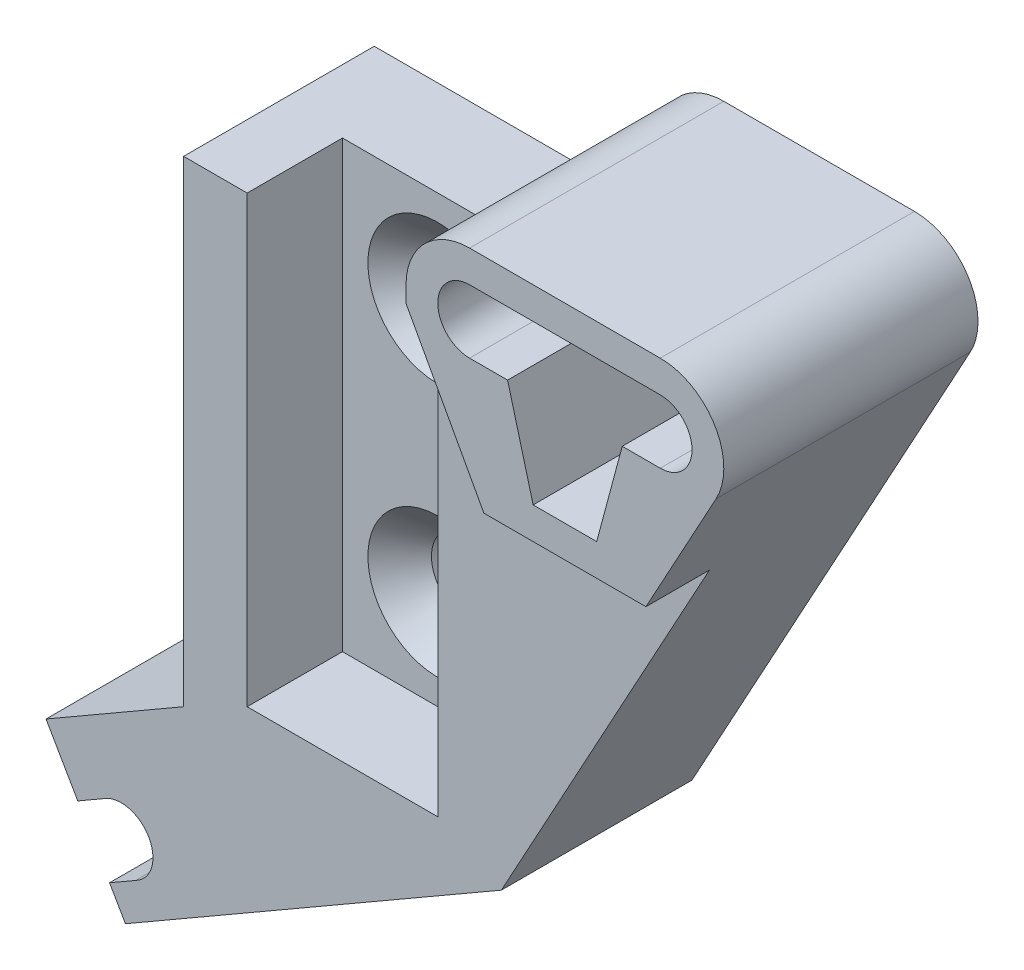
ISO-10303-21;
HEADER;
FILE_DESCRIPTION(('STEP AP214'),'2;1');
FILE_NAME('part.step','',(''),(''),'','','');
FILE_SCHEMA(('AUTOMOTIVE_DESIGN { 1 0 10303 214 1 1 1 1 }'));
ENDSEC;
DATA;
#1=APPLICATION_CONTEXT('core data for automotive mechanical design processes');
#2=APPLICATION_PROTOCOL_DEFINITION('international standard','automotive_design',2000,#1);
#3=PRODUCT_CONTEXT('',#1,'mechanical');
#4=PRODUCT('Part','Part','',(#3));
#5=PRODUCT_RELATED_PRODUCT_CATEGORY('part','',(#4));
#6=PRODUCT_DEFINITION_FORMATION('','',#4);
#7=PRODUCT_DEFINITION_CONTEXT('part definition',#1,'design');
#8=PRODUCT_DEFINITION('design','',#6,#7);
#9=PRODUCT_DEFINITION_SHAPE('','',#8);
#10=(LENGTH_UNIT() NAMED_UNIT(*) SI_UNIT(.MILLI.,.METRE.));
#11=(NAMED_UNIT(*) PLANE_ANGLE_UNIT() SI_UNIT($,.RADIAN.));
#12=(NAMED_UNIT(*) SI_UNIT($,.STERADIAN.) SOLID_ANGLE_UNIT());
#13=UNCERTAINTY_MEASURE_WITH_UNIT(LENGTH_MEASURE(1.E-05),#10,'distance_accuracy_value','');
#14=(GEOMETRIC_REPRESENTATION_CONTEXT(3) GLOBAL_UNCERTAINTY_ASSIGNED_CONTEXT((#13)) GLOBAL_UNIT_ASSIGNED_CONTEXT((#10,
#11,#12)) REPRESENTATION_CONTEXT('',''));
#15=CARTESIAN_POINT('',(0.,0.,0.));
#16=DIRECTION('',(0.,0.,1.));
#17=DIRECTION('',(1.,0.,0.));
#18=AXIS2_PLACEMENT_3D('',#15,#16,#17);
#19=CARTESIAN_POINT('',(17.0000000000015,16.9999999999993,6.));
#20=DIRECTION('',(0.,0.,-1.));
#21=DIRECTION('',(-1.,0.,0.));
#22=AXIS2_PLACEMENT_3D('',#19,#20,#21);
#23=CYLINDRICAL_SURFACE('',#22,0.999999999999349);
#24=CARTESIAN_POINT('',(17.0000000000015,16.9999999999993,0.));
#25=DIRECTION('',(0.,0.,1.));
#26=DIRECTION('',(1.,0.,0.));
#27=AXIS2_PLACEMENT_3D('',#24,#25,#26);
#28=CIRCLE('',#27,0.999999999999349);
#29=CARTESIAN_POINT('',(17.0000000000015,16.,0.));
#30=VERTEX_POINT('',#29);
#31=CARTESIAN_POINT('',(17.0000000000015,17.9999999999987,0.));
#32=VERTEX_POINT('',#31);
#33=EDGE_CURVE('E392',#30,#32,#28,.T.);
#34=ORIENTED_EDGE('',*,*,#33,.F.);
#35=DIRECTION('',(0.,0.,-1.));
#36=VECTOR('',#35,1.);
#37=CARTESIAN_POINT('',(17.0000000000015,16.,6.));
#38=LINE('',#37,#36);
#39=CARTESIAN_POINT('',(17.0000000000015,16.,8.));
#40=VERTEX_POINT('',#39);
#41=EDGE_CURVE('E11',#40,#30,#38,.T.);
#42=ORIENTED_EDGE('',*,*,#41,.F.);
#43=CARTESIAN_POINT('',(17.0000000000015,16.9999999999993,8.));
#44=DIRECTION('',(0.,0.,1.));
#45=DIRECTION('',(1.,0.,0.));
#46=AXIS2_PLACEMENT_3D('',#43,#44,#45);
#47=CIRCLE('',#46,0.999999999999349);
#48=CARTESIAN_POINT('',(17.0000000000015,17.9999999999987,8.));
#49=VERTEX_POINT('',#48);
#50=EDGE_CURVE('E285',#40,#49,#47,.T.);
#51=ORIENTED_EDGE('',*,*,#50,.T.);
#52=DIRECTION('',(0.,0.,-1.));
#53=VECTOR('',#52,1.);
#54=CARTESIAN_POINT('',(17.0000000000015,17.9999999999987,6.));
#55=LINE('',#54,#53);
#56=EDGE_CURVE('E413',#49,#32,#55,.T.);
#57=ORIENTED_EDGE('',*,*,#56,.T.);
#58=EDGE_LOOP('',(#34,#42,#51,#57));
#59=FACE_BOUND('',#58,.T.);
#60=ADVANCED_FACE('F50',(#59),#23,.F.);
#61=CARTESIAN_POINT('',(0.,16.,6.));
#62=DIRECTION('',(0.,-1.,0.));
#63=DIRECTION('',(0.,0.,-1.));
#64=AXIS2_PLACEMENT_3D('',#61,#62,#63);
#65=PLANE('',#64);
#66=DIRECTION('',(-1.,0.,0.));
#67=VECTOR('',#66,1.);
#68=CARTESIAN_POINT('',(0.,16.,0.));
#69=LINE('',#68,#67);
#70=CARTESIAN_POINT('',(15.8038475772934,16.,0.));
#71=VERTEX_POINT('',#70);
#72=EDGE_CURVE('E395',#30,#71,#69,.T.);
#73=ORIENTED_EDGE('',*,*,#72,.T.);
#74=DIRECTION('',(0.,0.,-1.));
#75=VECTOR('',#74,1.);
#76=CARTESIAN_POINT('',(15.8038475772934,16.,6.));
#77=LINE('',#76,#75);
#78=CARTESIAN_POINT('',(15.8038475772934,16.,8.));
#79=VERTEX_POINT('',#78);
#80=EDGE_CURVE('E57',#79,#71,#77,.T.);
#81=ORIENTED_EDGE('',*,*,#80,.F.);
#82=DIRECTION('',(1.,0.,0.));
#83=VECTOR('',#82,1.);
#84=CARTESIAN_POINT('',(15.8038475772934,16.,8.));
#85=LINE('',#84,#83);
#86=EDGE_CURVE('E282',#79,#40,#85,.T.);
#87=ORIENTED_EDGE('',*,*,#86,.T.);
#88=ORIENTED_EDGE('',*,*,#41,.T.);
#89=EDGE_LOOP('',(#73,#81,#87,#88));
#90=FACE_BOUND('',#89,.T.);
#91=ADVANCED_FACE('F530',(#90),#65,.F.);
#92=CARTESIAN_POINT('',(10.7451905283834,-2.87916512459883,6.));
#93=DIRECTION('',(-0.965925826289069,0.258819045102517,0.));
#94=DIRECTION('',(-0.258819045102517,-0.965925826289069,0.));
#95=AXIS2_PLACEMENT_3D('',#92,#93,#94);
#96=PLANE('',#95);
#97=DIRECTION('',(0.258819045102517,0.965925826289069,0.));
#98=VECTOR('',#97,1.);
#99=CARTESIAN_POINT('',(10.7451905283834,-2.87916512459883,0.));
#100=LINE('',#99,#98);
#101=CARTESIAN_POINT('',(15.,13.,0.));
#102=VERTEX_POINT('',#101);
#103=EDGE_CURVE('E399',#102,#71,#100,.T.);
#104=ORIENTED_EDGE('',*,*,#103,.F.);
#105=DIRECTION('',(0.,0.,-1.));
#106=VECTOR('',#105,1.);
#107=CARTESIAN_POINT('',(15.,13.,6.));
#108=LINE('',#107,#106);
#109=CARTESIAN_POINT('',(15.,13.,8.));
#110=VERTEX_POINT('',#109);
#111=EDGE_CURVE('E426',#110,#102,#108,.T.);
#112=ORIENTED_EDGE('',*,*,#111,.F.);
#113=DIRECTION('',(0.258819045102517,0.965925826289069,0.));
#114=VECTOR('',#113,1.);
#115=CARTESIAN_POINT('',(15.8038475772934,16.,8.));
#116=LINE('',#115,#114);
#117=EDGE_CURVE('E276',#110,#79,#116,.T.);
#118=ORIENTED_EDGE('',*,*,#117,.T.);
#119=ORIENTED_EDGE('',*,*,#80,.T.);
#120=EDGE_LOOP('',(#104,#112,#118,#119));
#121=FACE_BOUND('',#120,.T.);
#122=ADVANCED_FACE('F532',(#121),#96,.T.);
#123=CARTESIAN_POINT('',(0.,13.,6.));
#124=DIRECTION('',(0.,1.,0.));
#125=DIRECTION('',(0.,0.,1.));
#126=AXIS2_PLACEMENT_3D('',#123,#124,#125);
#127=PLANE('',#126);
#128=DIRECTION('',(1.,0.,0.));
#129=VECTOR('',#128,1.);
#130=CARTESIAN_POINT('',(0.,13.,0.));
#131=LINE('',#130,#129);
#132=CARTESIAN_POINT('',(13.,13.,0.));
#133=VERTEX_POINT('',#132);
#134=EDGE_CURVE('E402',#133,#102,#131,.T.);
#135=ORIENTED_EDGE('',*,*,#134,.F.);
#136=DIRECTION('',(0.,0.,-1.));
#137=VECTOR('',#136,1.);
#138=CARTESIAN_POINT('',(13.,13.,6.));
#139=LINE('',#138,#137);
#140=CARTESIAN_POINT('',(13.,13.,8.));
#141=VERTEX_POINT('',#140);
#142=EDGE_CURVE('E424',#141,#133,#139,.T.);
#143=ORIENTED_EDGE('',*,*,#142,.F.);
#144=DIRECTION('',(1.,0.,0.));
#145=VECTOR('',#144,1.);
#146=CARTESIAN_POINT('',(15.,13.,8.));
#147=LINE('',#146,#145);
#148=EDGE_CURVE('E277',#141,#110,#147,.T.);
#149=ORIENTED_EDGE('',*,*,#148,.T.);
#150=ORIENTED_EDGE('',*,*,#111,.T.);
#151=EDGE_LOOP('',(#135,#143,#149,#150));
#152=FACE_BOUND('',#151,.T.);
#153=ADVANCED_FACE('F770',(#152),#127,.T.);
#154=CARTESIAN_POINT('',(15.3791651245988,4.12083487540106,6.));
#155=DIRECTION('',(-0.96592582628907,-0.258819045102516,0.));
#156=DIRECTION('',(0.258819045102516,-0.96592582628907,0.));
#157=AXIS2_PLACEMENT_3D('',#154,#155,#156);
#158=PLANE('',#157);
#159=DIRECTION('',(-0.258819045102516,0.96592582628907,0.));
#160=VECTOR('',#159,1.);
#161=CARTESIAN_POINT('',(15.3791651245988,4.12083487540106,0.));
#162=LINE('',#161,#160);
#163=CARTESIAN_POINT('',(12.1961524227066,16.,0.));
#164=VERTEX_POINT('',#163);
#165=EDGE_CURVE('E404',#133,#164,#162,.T.);
#166=ORIENTED_EDGE('',*,*,#165,.T.);
#167=DIRECTION('',(0.,0.,-1.));
#168=VECTOR('',#167,1.);
#169=CARTESIAN_POINT('',(12.1961524227066,16.,6.));
#170=LINE('',#169,#168);
#171=CARTESIAN_POINT('',(12.1961524227066,16.,8.));
#172=VERTEX_POINT('',#171);
#173=EDGE_CURVE('E423',#172,#164,#170,.T.);
#174=ORIENTED_EDGE('',*,*,#173,.F.);
#175=DIRECTION('',(0.258819045102516,-0.965925826289069,0.));
#176=VECTOR('',#175,1.);
#177=CARTESIAN_POINT('',(13.,13.,8.));
#178=LINE('',#177,#176);
#179=EDGE_CURVE('E272',#172,#141,#178,.T.);
#180=ORIENTED_EDGE('',*,*,#179,.T.);
#181=ORIENTED_EDGE('',*,*,#142,.T.);
#182=EDGE_LOOP('',(#166,#174,#180,#181));
#183=FACE_BOUND('',#182,.T.);
#184=ADVANCED_FACE('F760',(#183),#158,.F.);
#185=CARTESIAN_POINT('',(0.,16.,6.));
#186=DIRECTION('',(0.,-1.,0.));
#187=DIRECTION('',(0.,0.,-1.));
#188=AXIS2_PLACEMENT_3D('',#185,#186,#187);
#189=PLANE('',#188);
#190=DIRECTION('',(-1.,0.,0.));
#191=VECTOR('',#190,1.);
#192=CARTESIAN_POINT('',(0.,16.,0.));
#193=LINE('',#192,#191);
#194=CARTESIAN_POINT('',(11.,16.,0.));
#195=VERTEX_POINT('',#194);
#196=EDGE_CURVE('E407',#164,#195,#193,.T.);
#197=ORIENTED_EDGE('',*,*,#196,.T.);
#198=DIRECTION('',(0.,0.,-1.));
#199=VECTOR('',#198,1.);
#200=CARTESIAN_POINT('',(11.,16.,6.));
#201=LINE('',#200,#199);
#202=CARTESIAN_POINT('',(11.,16.,8.));
#203=VERTEX_POINT('',#202);
#204=EDGE_CURVE('E420',#203,#195,#201,.T.);
#205=ORIENTED_EDGE('',*,*,#204,.F.);
#206=DIRECTION('',(1.,0.,0.));
#207=VECTOR('',#206,1.);
#208=CARTESIAN_POINT('',(11.,16.,8.));
#209=LINE('',#208,#207);
#210=EDGE_CURVE('E267',#203,#172,#209,.T.);
#211=ORIENTED_EDGE('',*,*,#210,.T.);
#212=ORIENTED_EDGE('',*,*,#173,.T.);
#213=EDGE_LOOP('',(#197,#205,#211,#212));
#214=FACE_BOUND('',#213,.T.);
#215=ADVANCED_FACE('F747',(#214),#189,.F.);
#216=CARTESIAN_POINT('',(11.,16.9999999999995,6.));
#217=DIRECTION('',(0.,0.,-1.));
#218=DIRECTION('',(-1.,0.,0.));
#219=AXIS2_PLACEMENT_3D('',#216,#217,#218);
#220=CYLINDRICAL_SURFACE('',#219,0.99999999999934);
#221=CARTESIAN_POINT('',(11.,16.9999999999995,0.));
#222=DIRECTION('',(0.,0.,1.));
#223=DIRECTION('',(1.,0.,0.));
#224=AXIS2_PLACEMENT_3D('',#221,#222,#223);
#225=CIRCLE('',#224,0.99999999999934);
#226=CARTESIAN_POINT('',(11.,17.9999999999987,0.));
#227=VERTEX_POINT('',#226);
#228=EDGE_CURVE('E410',#227,#195,#225,.T.);
#229=ORIENTED_EDGE('',*,*,#228,.F.);
#230=DIRECTION('',(0.,0.,-1.));
#231=VECTOR('',#230,1.);
#232=CARTESIAN_POINT('',(11.,17.9999999999987,6.));
#233=LINE('',#232,#231);
#234=CARTESIAN_POINT('',(11.,17.9999999999987,8.));
#235=VERTEX_POINT('',#234);
#236=EDGE_CURVE('E417',#235,#227,#233,.T.);
#237=ORIENTED_EDGE('',*,*,#236,.F.);
#238=CARTESIAN_POINT('',(11.,16.9999999999995,8.));
#239=DIRECTION('',(0.,0.,1.));
#240=DIRECTION('',(1.,0.,0.));
#241=AXIS2_PLACEMENT_3D('',#238,#239,#240);
#242=CIRCLE('',#241,0.99999999999934);
#243=EDGE_CURVE('E266',#235,#203,#242,.T.);
#244=ORIENTED_EDGE('',*,*,#243,.T.);
#245=ORIENTED_EDGE('',*,*,#204,.T.);
#246=EDGE_LOOP('',(#229,#237,#244,#245));
#247=FACE_BOUND('',#246,.T.);
#248=ADVANCED_FACE('F741',(#247),#220,.F.);
#249=CARTESIAN_POINT('',(7.70480572843409,-4.20523792090649,6.));
#250=DIRECTION('',(0.877770227817856,-0.479081858513333,0.));
#251=DIRECTION('',(0.479081858513333,0.877770227817856,0.));
#252=AXIS2_PLACEMENT_3D('',#249,#250,#251);
#253=PLANE('',#252);
#254=DIRECTION('',(-0.479081858513333,-0.877770227817856,0.));
#255=VECTOR('',#254,1.);
#256=CARTESIAN_POINT('',(7.70480572843409,-4.20523792090649,0.));
#257=LINE('',#256,#255);
#258=CARTESIAN_POINT('',(18.7555404556372,16.0418362829727,0.));
#259=VERTEX_POINT('',#258);
#260=CARTESIAN_POINT('',(9.99999999999997,0.,0.));
#261=VERTEX_POINT('',#260);
#262=EDGE_CURVE('E325',#259,#261,#257,.T.);
#263=ORIENTED_EDGE('',*,*,#262,.F.);
#264=DIRECTION('',(0.,0.,-1.));
#265=VECTOR('',#264,1.);
#266=CARTESIAN_POINT('',(18.7555404556372,16.0418362829727,6.));
#267=LINE('',#266,#265);
#268=CARTESIAN_POINT('',(18.7555404556372,16.0418362829727,8.));
#269=VERTEX_POINT('',#268);
#270=EDGE_CURVE('E51',#269,#259,#267,.T.);
#271=ORIENTED_EDGE('',*,*,#270,.F.);
#272=DIRECTION('',(0.479081858513333,0.877770227817856,0.));
#273=VECTOR('',#272,1.);
#274=CARTESIAN_POINT('',(16.549529842738,12.,8.));
#275=LINE('',#274,#273);
#276=CARTESIAN_POINT('',(16.549529842738,12.,8.));
#277=VERTEX_POINT('',#276);
#278=EDGE_CURVE('E307',#277,#269,#275,.T.);
#279=ORIENTED_EDGE('',*,*,#278,.F.);
#280=DIRECTION('',(0.,0.,-1.));
#281=VECTOR('',#280,1.);
#282=CARTESIAN_POINT('',(16.549529842738,12.,8.));
#283=LINE('',#282,#281);
#284=CARTESIAN_POINT('',(16.549529842738,12.,6.));
#285=VERTEX_POINT('',#284);
#286=EDGE_CURVE('E309',#277,#285,#283,.T.);
#287=ORIENTED_EDGE('',*,*,#286,.T.);
#288=DIRECTION('',(-0.479081858513333,-0.877770227817856,0.));
#289=VECTOR('',#288,1.);
#290=CARTESIAN_POINT('',(7.70480572843409,-4.20523792090649,6.));
#291=LINE('',#290,#289);
#292=CARTESIAN_POINT('',(9.99999999999997,0.,6.));
#293=VERTEX_POINT('',#292);
#294=EDGE_CURVE('E323',#285,#293,#291,.T.);
#295=ORIENTED_EDGE('',*,*,#294,.T.);
#296=DIRECTION('',(0.,0.,-1.));
#297=VECTOR('',#296,1.);
#298=CARTESIAN_POINT('',(9.99999999999997,0.,6.));
#299=LINE('',#298,#297);
#300=EDGE_CURVE('E352',#293,#261,#299,.T.);
#301=ORIENTED_EDGE('',*,*,#300,.T.);
#302=EDGE_LOOP('',(#263,#271,#279,#287,#295,#301));
#303=FACE_BOUND('',#302,.T.);
#304=ADVANCED_FACE('F47',(#303),#253,.T.);
#305=CARTESIAN_POINT('',(17.0000000000015,16.9999999999993,6.));
#306=DIRECTION('',(0.,0.,-1.));
#307=DIRECTION('',(-1.,0.,0.));
#308=AXIS2_PLACEMENT_3D('',#305,#306,#307);
#309=CYLINDRICAL_SURFACE('',#308,2.);
#310=CARTESIAN_POINT('',(17.0000000000015,16.9999999999993,0.));
#311=DIRECTION('',(0.,0.,1.));
#312=DIRECTION('',(1.,0.,0.));
#313=AXIS2_PLACEMENT_3D('',#310,#311,#312);
#314=CIRCLE('',#313,2.);
#315=CARTESIAN_POINT('',(17.0000000000015,18.9999999999993,0.));
#316=VERTEX_POINT('',#315);
#317=EDGE_CURVE('E355',#259,#316,#314,.T.);
#318=ORIENTED_EDGE('',*,*,#317,.T.);
#319=DIRECTION('',(0.,0.,-1.));
#320=VECTOR('',#319,1.);
#321=CARTESIAN_POINT('',(17.0000000000015,18.9999999999993,6.));
#322=LINE('',#321,#320);
#323=CARTESIAN_POINT('',(17.0000000000015,18.9999999999993,8.));
#324=VERTEX_POINT('',#323);
#325=EDGE_CURVE('E454',#324,#316,#322,.T.);
#326=ORIENTED_EDGE('',*,*,#325,.F.);
#327=CARTESIAN_POINT('',(17.0000000000015,16.9999999999993,8.));
#328=DIRECTION('',(0.,0.,1.));
#329=DIRECTION('',(1.,0.,0.));
#330=AXIS2_PLACEMENT_3D('',#327,#328,#329);
#331=CIRCLE('',#330,2.00000000000001);
#332=EDGE_CURVE('E292',#269,#324,#331,.T.);
#333=ORIENTED_EDGE('',*,*,#332,.F.);
#334=ORIENTED_EDGE('',*,*,#270,.T.);
#335=EDGE_LOOP('',(#318,#326,#333,#334));
#336=FACE_BOUND('',#335,.T.);
#337=ADVANCED_FACE('F458',(#336),#309,.T.);
#338=CARTESIAN_POINT('',(4.61436444609707E-13,18.9999999999998,6.));
#339=DIRECTION('',(0.,1.,0.));
#340=DIRECTION('',(-1.,0.,0.));
#341=AXIS2_PLACEMENT_3D('',#338,#339,#340);
#342=PLANE('',#341);
#343=DIRECTION('',(1.,0.,0.));
#344=VECTOR('',#343,1.);
#345=CARTESIAN_POINT('',(4.61436444609707E-13,18.9999999999998,0.));
#346=LINE('',#345,#344);
#347=CARTESIAN_POINT('',(11.,18.9999999999995,0.));
#348=VERTEX_POINT('',#347);
#349=EDGE_CURVE('E359',#348,#316,#346,.T.);
#350=ORIENTED_EDGE('',*,*,#349,.F.);
#351=DIRECTION('',(0.,0.,-1.));
#352=VECTOR('',#351,1.);
#353=CARTESIAN_POINT('',(11.,18.9999999999995,6.));
#354=LINE('',#353,#352);
#355=CARTESIAN_POINT('',(11.,18.9999999999995,8.));
#356=VERTEX_POINT('',#355);
#357=EDGE_CURVE('E455',#356,#348,#354,.T.);
#358=ORIENTED_EDGE('',*,*,#357,.F.);
#359=DIRECTION('',(-1.,0.,0.));
#360=VECTOR('',#359,1.);
#361=CARTESIAN_POINT('',(17.0000000000015,18.9999999999993,8.));
#362=LINE('',#361,#360);
#363=EDGE_CURVE('E294',#324,#356,#362,.T.);
#364=ORIENTED_EDGE('',*,*,#363,.F.);
#365=ORIENTED_EDGE('',*,*,#325,.T.);
#366=EDGE_LOOP('',(#350,#358,#364,#365));
#367=FACE_BOUND('',#366,.T.);
#368=ADVANCED_FACE('F520',(#367),#342,.T.);
#369=CARTESIAN_POINT('',(11.,16.9999999999995,6.));
#370=DIRECTION('',(0.,0.,-1.));
#371=DIRECTION('',(-1.,0.,0.));
#372=AXIS2_PLACEMENT_3D('',#369,#370,#371);
#373=CYLINDRICAL_SURFACE('',#372,2.);
#374=CARTESIAN_POINT('',(11.,16.9999999999995,0.));
#375=DIRECTION('',(0.,0.,1.));
#376=DIRECTION('',(1.,0.,0.));
#377=AXIS2_PLACEMENT_3D('',#374,#375,#376);
#378=CIRCLE('',#377,2.);
#379=CARTESIAN_POINT('',(9.,16.9999999999995,0.));
#380=VERTEX_POINT('',#379);
#381=EDGE_CURVE('E363',#348,#380,#378,.T.);
#382=ORIENTED_EDGE('',*,*,#381,.T.);
#383=DIRECTION('',(0.,0.,-1.));
#384=VECTOR('',#383,1.);
#385=CARTESIAN_POINT('',(9.,16.9999999999995,6.));
#386=LINE('',#385,#384);
#387=CARTESIAN_POINT('',(9.,16.9999999999995,8.));
#388=VERTEX_POINT('',#387);
#389=EDGE_CURVE('E448',#388,#380,#386,.T.);
#390=ORIENTED_EDGE('',*,*,#389,.F.);
#391=CARTESIAN_POINT('',(11.,16.9999999999995,8.));
#392=DIRECTION('',(0.,0.,1.));
#393=DIRECTION('',(1.,0.,0.));
#394=AXIS2_PLACEMENT_3D('',#391,#392,#393);
#395=CIRCLE('',#394,2.);
#396=EDGE_CURVE('E299',#356,#388,#395,.T.);
#397=ORIENTED_EDGE('',*,*,#396,.F.);
#398=ORIENTED_EDGE('',*,*,#357,.T.);
#399=EDGE_LOOP('',(#382,#390,#397,#398));
#400=FACE_BOUND('',#399,.T.);
#401=ADVANCED_FACE('F516',(#400),#373,.T.);
#402=CARTESIAN_POINT('',(9.,0.,6.));
#403=DIRECTION('',(1.,0.,0.));
#404=DIRECTION('',(0.,0.,-1.));
#405=AXIS2_PLACEMENT_3D('',#402,#403,#404);
#406=PLANE('',#405);
#407=DIRECTION('',(0.,-1.,0.));
#408=VECTOR('',#407,1.);
#409=CARTESIAN_POINT('',(9.,0.,0.));
#410=LINE('',#409,#408);
#411=CARTESIAN_POINT('',(9.,15.,0.));
#412=VERTEX_POINT('',#411);
#413=EDGE_CURVE('E361',#380,#412,#410,.T.);
#414=ORIENTED_EDGE('',*,*,#413,.T.);
#415=DIRECTION('',(0.,0.,-1.));
#416=VECTOR('',#415,1.);
#417=CARTESIAN_POINT('',(9.,15.,6.));
#418=LINE('',#417,#416);
#419=CARTESIAN_POINT('',(9.,15.,6.));
#420=VERTEX_POINT('',#419);
#421=EDGE_CURVE('E447',#420,#412,#418,.T.);
#422=ORIENTED_EDGE('',*,*,#421,.F.);
#423=DIRECTION('',(0.,-1.,0.));
#424=VECTOR('',#423,1.);
#425=CARTESIAN_POINT('',(9.,0.,6.));
#426=LINE('',#425,#424);
#427=CARTESIAN_POINT('',(9.,16.4897332469976,6.));
#428=VERTEX_POINT('',#427);
#429=EDGE_CURVE('E324',#428,#420,#426,.T.);
#430=ORIENTED_EDGE('',*,*,#429,.F.);
#431=DIRECTION('',(0.,0.,-1.));
#432=VECTOR('',#431,1.);
#433=CARTESIAN_POINT('',(9.,16.4897332469976,8.));
#434=LINE('',#433,#432);
#435=CARTESIAN_POINT('',(9.,16.4897332469976,8.));
#436=VERTEX_POINT('',#435);
#437=EDGE_CURVE('E317',#436,#428,#434,.T.);
#438=ORIENTED_EDGE('',*,*,#437,.F.);
#439=DIRECTION('',(0.,-1.,0.));
#440=VECTOR('',#439,1.);
#441=CARTESIAN_POINT('',(9.,16.9999999999995,8.));
#442=LINE('',#441,#440);
#443=EDGE_CURVE('E302',#388,#436,#442,.T.);
#444=ORIENTED_EDGE('',*,*,#443,.F.);
#445=ORIENTED_EDGE('',*,*,#389,.T.);
#446=EDGE_LOOP('',(#414,#422,#430,#438,#444,#445));
#447=FACE_BOUND('',#446,.T.);
#448=ADVANCED_FACE('F512',(#447),#406,.F.);
#449=CARTESIAN_POINT('',(0.,15.,6.));
#450=DIRECTION('',(0.,1.,0.));
#451=DIRECTION('',(0.,0.,1.));
#452=AXIS2_PLACEMENT_3D('',#449,#450,#451);
#453=PLANE('',#452);
#454=DIRECTION('',(0.,0.,1.));
#455=VECTOR('',#454,1.);
#456=CARTESIAN_POINT('',(2.,15.,0.));
#457=LINE('',#456,#455);
#458=CARTESIAN_POINT('',(2.,15.,3.));
#459=VERTEX_POINT('',#458);
#460=CARTESIAN_POINT('',(2.,15.,6.));
#461=VERTEX_POINT('',#460);
#462=EDGE_CURVE('E254',#459,#461,#457,.T.);
#463=ORIENTED_EDGE('',*,*,#462,.F.);
#464=DIRECTION('',(1.,0.,0.));
#465=VECTOR('',#464,1.);
#466=CARTESIAN_POINT('',(0.,15.,3.));
#467=LINE('',#466,#465);
#468=CARTESIAN_POINT('',(8.,15.,3.));
#469=VERTEX_POINT('',#468);
#470=EDGE_CURVE('E1017',#459,#469,#467,.T.);
#471=ORIENTED_EDGE('',*,*,#470,.T.);
#472=DIRECTION('',(0.,0.,-1.));
#473=VECTOR('',#472,1.);
#474=CARTESIAN_POINT('',(8.,15.,0.));
#475=LINE('',#474,#473);
#476=CARTESIAN_POINT('',(8.,15.,6.));
#477=VERTEX_POINT('',#476);
#478=EDGE_CURVE('E1012',#477,#469,#475,.T.);
#479=ORIENTED_EDGE('',*,*,#478,.F.);
#480=DIRECTION('',(1.,0.,0.));
#481=VECTOR('',#480,1.);
#482=CARTESIAN_POINT('',(0.,15.,6.));
#483=LINE('',#482,#481);
#484=EDGE_CURVE('E259',#477,#420,#483,.T.);
#485=ORIENTED_EDGE('',*,*,#484,.T.);
#486=ORIENTED_EDGE('',*,*,#421,.T.);
#487=DIRECTION('',(1.,0.,0.));
#488=VECTOR('',#487,1.);
#489=CARTESIAN_POINT('',(0.,15.,0.));
#490=LINE('',#489,#488);
#491=CARTESIAN_POINT('',(0.,15.,0.));
#492=VERTEX_POINT('',#491);
#493=EDGE_CURVE('E368',#492,#412,#490,.T.);
#494=ORIENTED_EDGE('',*,*,#493,.F.);
#495=DIRECTION('',(0.,0.,-1.));
#496=VECTOR('',#495,1.);
#497=CARTESIAN_POINT('',(0.,15.,6.));
#498=LINE('',#497,#496);
#499=CARTESIAN_POINT('',(0.,15.,6.));
#500=VERTEX_POINT('',#499);
#501=EDGE_CURVE('E443',#500,#492,#498,.T.);
#502=ORIENTED_EDGE('',*,*,#501,.F.);
#503=EDGE_CURVE('E327',#500,#461,#483,.T.);
#504=ORIENTED_EDGE('',*,*,#503,.T.);
#505=EDGE_LOOP('',(#463,#471,#479,#485,#486,#494,#502,#504));
#506=FACE_BOUND('',#505,.T.);
#507=ADVANCED_FACE('F510',(#506),#453,.T.);
#508=CARTESIAN_POINT('',(0.,0.,6.));
#509=DIRECTION('',(-1.,0.,0.));
#510=DIRECTION('',(0.,0.,1.));
#511=AXIS2_PLACEMENT_3D('',#508,#509,#510);
#512=PLANE('',#511);
#513=DIRECTION('',(0.,1.,0.));
#514=VECTOR('',#513,1.);
#515=CARTESIAN_POINT('',(0.,0.,0.));
#516=LINE('',#515,#514);
#517=CARTESIAN_POINT('',(0.,0.,0.));
#518=VERTEX_POINT('',#517);
#519=EDGE_CURVE('E369',#518,#492,#516,.T.);
#520=ORIENTED_EDGE('',*,*,#519,.F.);
#521=DIRECTION('',(0.,0.,-1.));
#522=VECTOR('',#521,1.);
#523=CARTESIAN_POINT('',(0.,0.,6.));
#524=LINE('',#523,#522);
#525=CARTESIAN_POINT('',(0.,0.,6.));
#526=VERTEX_POINT('',#525);
#527=EDGE_CURVE('E444',#526,#518,#524,.T.);
#528=ORIENTED_EDGE('',*,*,#527,.F.);
#529=DIRECTION('',(0.,1.,0.));
#530=VECTOR('',#529,1.);
#531=CARTESIAN_POINT('',(0.,0.,6.));
#532=LINE('',#531,#530);
#533=EDGE_CURVE('E332',#526,#500,#532,.T.);
#534=ORIENTED_EDGE('',*,*,#533,.T.);
#535=ORIENTED_EDGE('',*,*,#501,.T.);
#536=EDGE_LOOP('',(#520,#528,#534,#535));
#537=FACE_BOUND('',#536,.T.);
#538=ADVANCED_FACE('F502',(#537),#512,.T.);
#539=CARTESIAN_POINT('',(0.,0.,6.));
#540=DIRECTION('',(0.499999999999995,-0.866025403784441,0.));
#541=DIRECTION('',(0.866025403784441,0.499999999999995,0.));
#542=AXIS2_PLACEMENT_3D('',#539,#540,#541);
#543=PLANE('',#542);
#544=DIRECTION('',(-0.866025403784441,-0.499999999999995,0.));
#545=VECTOR('',#544,1.);
#546=CARTESIAN_POINT('',(0.,0.,0.));
#547=LINE('',#546,#545);
#548=CARTESIAN_POINT('',(-4.33012701892221,-2.49999999999998,0.));
#549=VERTEX_POINT('',#548);
#550=EDGE_CURVE('E375',#518,#549,#547,.T.);
#551=ORIENTED_EDGE('',*,*,#550,.T.);
#552=DIRECTION('',(0.,0.,-1.));
#553=VECTOR('',#552,1.);
#554=CARTESIAN_POINT('',(-4.33012701892221,-2.49999999999998,6.));
#555=LINE('',#554,#553);
#556=CARTESIAN_POINT('',(-4.33012701892221,-2.49999999999998,6.));
#557=VERTEX_POINT('',#556);
#558=EDGE_CURVE('E439',#557,#549,#555,.T.);
#559=ORIENTED_EDGE('',*,*,#558,.F.);
#560=DIRECTION('',(-0.866025403784441,-0.499999999999995,0.));
#561=VECTOR('',#560,1.);
#562=CARTESIAN_POINT('',(0.,0.,6.));
#563=LINE('',#562,#561);
#564=EDGE_CURVE('E331',#526,#557,#563,.T.);
#565=ORIENTED_EDGE('',*,*,#564,.F.);
#566=ORIENTED_EDGE('',*,*,#527,.T.);
#567=EDGE_LOOP('',(#551,#559,#565,#566));
#568=FACE_BOUND('',#567,.T.);
#569=ADVANCED_FACE('F496',(#568),#543,.F.);
#570=CARTESIAN_POINT('',(-4.33012701892221,-2.49999999999998,6.));
#571=DIRECTION('',(0.866025403784441,0.499999999999995,0.));
#572=DIRECTION('',(-0.499999999999995,0.866025403784441,0.));
#573=AXIS2_PLACEMENT_3D('',#570,#571,#572);
#574=PLANE('',#573);
#575=DIRECTION('',(0.499999999999995,-0.866025403784441,0.));
#576=VECTOR('',#575,1.);
#577=CARTESIAN_POINT('',(-4.33012701892221,-2.49999999999998,0.));
#578=LINE('',#577,#576);
#579=CARTESIAN_POINT('',(-3.32956964541445,-4.2330162068031,0.));
#580=VERTEX_POINT('',#579);
#581=EDGE_CURVE('E372',#549,#580,#578,.T.);
#582=ORIENTED_EDGE('',*,*,#581,.T.);
#583=DIRECTION('',(0.,0.,-1.));
#584=VECTOR('',#583,1.);
#585=CARTESIAN_POINT('',(-3.32956964541445,-4.2330162068031,6.));
#586=LINE('',#585,#584);
#587=CARTESIAN_POINT('',(-3.32956964541445,-4.2330162068031,6.));
#588=VERTEX_POINT('',#587);
#589=EDGE_CURVE('E437',#588,#580,#586,.T.);
#590=ORIENTED_EDGE('',*,*,#589,.F.);
#591=DIRECTION('',(0.499999999999995,-0.866025403784441,0.));
#592=VECTOR('',#591,1.);
#593=CARTESIAN_POINT('',(-4.33012701892221,-2.49999999999998,6.));
#594=LINE('',#593,#592);
#595=EDGE_CURVE('E336',#557,#588,#594,.T.);
#596=ORIENTED_EDGE('',*,*,#595,.F.);
#597=ORIENTED_EDGE('',*,*,#558,.T.);
#598=EDGE_LOOP('',(#582,#590,#596,#597));
#599=FACE_BOUND('',#598,.T.);
#600=ADVANCED_FACE('F493',(#599),#574,.F.);
#601=CARTESIAN_POINT('',(1.00055737350775,-1.73301620680312,6.));
#602=DIRECTION('',(0.499999999999996,-0.866025403784441,0.));
#603=DIRECTION('',(0.866025403784441,0.499999999999996,0.));
#604=AXIS2_PLACEMENT_3D('',#601,#602,#603);
#605=PLANE('',#604);
#606=DIRECTION('',(-0.866025403784441,-0.499999999999996,0.));
#607=VECTOR('',#606,1.);
#608=CARTESIAN_POINT('',(1.00055737350775,-1.73301620680312,0.));
#609=LINE('',#608,#607);
#610=CARTESIAN_POINT('',(-2.50442441442294,-3.75661838556962,0.));
#611=VERTEX_POINT('',#610);
#612=EDGE_CURVE('E380',#611,#580,#609,.T.);
#613=ORIENTED_EDGE('',*,*,#612,.F.);
#614=DIRECTION('',(0.,0.,-1.));
#615=VECTOR('',#614,1.);
#616=CARTESIAN_POINT('',(-2.50442441442294,-3.75661838556962,6.));
#617=LINE('',#616,#615);
#618=CARTESIAN_POINT('',(-2.50442441442294,-3.75661838556962,6.));
#619=VERTEX_POINT('',#618);
#620=EDGE_CURVE('E436',#619,#611,#617,.T.);
#621=ORIENTED_EDGE('',*,*,#620,.F.);
#622=DIRECTION('',(-0.866025403784441,-0.499999999999996,0.));
#623=VECTOR('',#622,1.);
#624=CARTESIAN_POINT('',(1.00055737350775,-1.73301620680312,6.));
#625=LINE('',#624,#623);
#626=EDGE_CURVE('E339',#619,#588,#625,.T.);
#627=ORIENTED_EDGE('',*,*,#626,.T.);
#628=ORIENTED_EDGE('',*,*,#589,.T.);
#629=EDGE_LOOP('',(#613,#621,#627,#628));
#630=FACE_BOUND('',#629,.T.);
#631=ADVANCED_FACE('F488',(#630),#605,.T.);
#632=CARTESIAN_POINT('',(-1.96410161513775,-4.59807621135332,6.));
#633=DIRECTION('',(0.,0.,-1.));
#634=DIRECTION('',(-1.,0.,0.));
#635=AXIS2_PLACEMENT_3D('',#632,#633,#634);
#636=CYLINDRICAL_SURFACE('',#635,1.);
#637=CARTESIAN_POINT('',(-1.96410161513775,-4.59807621135332,0.));
#638=DIRECTION('',(0.,0.,1.));
#639=DIRECTION('',(1.,0.,0.));
#640=AXIS2_PLACEMENT_3D('',#637,#638,#639);
#641=CIRCLE('',#640,1.);
#642=CARTESIAN_POINT('',(-1.50553916143826,-5.48673839466996,0.));
#643=VERTEX_POINT('',#642);
#644=EDGE_CURVE('E379',#643,#611,#641,.T.);
#645=ORIENTED_EDGE('',*,*,#644,.F.);
#646=DIRECTION('',(0.,0.,-1.));
#647=VECTOR('',#646,1.);
#648=CARTESIAN_POINT('',(-1.50553916143826,-5.48673839466996,6.));
#649=LINE('',#648,#647);
#650=CARTESIAN_POINT('',(-1.50553916143826,-5.48673839466996,6.));
#651=VERTEX_POINT('',#650);
#652=EDGE_CURVE('E432',#651,#643,#649,.T.);
#653=ORIENTED_EDGE('',*,*,#652,.F.);
#654=CARTESIAN_POINT('',(-1.96410161513775,-4.59807621135332,6.));
#655=DIRECTION('',(0.,0.,1.));
#656=DIRECTION('',(1.,0.,0.));
#657=AXIS2_PLACEMENT_3D('',#654,#655,#656);
#658=CIRCLE('',#657,1.);
#659=EDGE_CURVE('E342',#651,#619,#658,.T.);
#660=ORIENTED_EDGE('',*,*,#659,.T.);
#661=ORIENTED_EDGE('',*,*,#620,.T.);
#662=EDGE_LOOP('',(#645,#653,#660,#661));
#663=FACE_BOUND('',#662,.T.);
#664=ADVANCED_FACE('F482',(#663),#636,.F.);
#665=CARTESIAN_POINT('',(1.99944262649224,-3.46313621590357,6.));
#666=DIRECTION('',(0.499999999999995,-0.866025403784441,0.));
#667=DIRECTION('',(0.866025403784441,0.499999999999995,0.));
#668=AXIS2_PLACEMENT_3D('',#665,#666,#667);
#669=PLANE('',#668);
#670=DIRECTION('',(-0.866025403784441,-0.499999999999995,0.));
#671=VECTOR('',#670,1.);
#672=CARTESIAN_POINT('',(1.99944262649224,-3.46313621590357,0.));
#673=LINE('',#672,#671);
#674=CARTESIAN_POINT('',(-2.33068439242996,-5.96313621590355,0.));
#675=VERTEX_POINT('',#674);
#676=EDGE_CURVE('E382',#643,#675,#673,.T.);
#677=ORIENTED_EDGE('',*,*,#676,.T.);
#678=DIRECTION('',(0.,0.,-1.));
#679=VECTOR('',#678,1.);
#680=CARTESIAN_POINT('',(-2.33068439242996,-5.96313621590355,6.));
#681=LINE('',#680,#679);
#682=CARTESIAN_POINT('',(-2.33068439242996,-5.96313621590355,6.));
#683=VERTEX_POINT('',#682);
#684=EDGE_CURVE('E435',#683,#675,#681,.T.);
#685=ORIENTED_EDGE('',*,*,#684,.F.);
#686=DIRECTION('',(-0.866025403784441,-0.499999999999995,0.));
#687=VECTOR('',#686,1.);
#688=CARTESIAN_POINT('',(1.99944262649224,-3.46313621590357,6.));
#689=LINE('',#688,#687);
#690=EDGE_CURVE('E341',#651,#683,#689,.T.);
#691=ORIENTED_EDGE('',*,*,#690,.F.);
#692=ORIENTED_EDGE('',*,*,#652,.T.);
#693=EDGE_LOOP('',(#677,#685,#691,#692));
#694=FACE_BOUND('',#693,.T.);
#695=ADVANCED_FACE('F546',(#694),#669,.F.);
#696=CARTESIAN_POINT('',(-4.33012701892221,-2.49999999999998,6.));
#697=DIRECTION('',(-0.866025403784441,-0.499999999999995,0.));
#698=DIRECTION('',(0.499999999999995,-0.866025403784441,0.));
#699=AXIS2_PLACEMENT_3D('',#696,#697,#698);
#700=PLANE('',#699);
#701=DIRECTION('',(-0.499999999999995,0.866025403784441,0.));
#702=VECTOR('',#701,1.);
#703=CARTESIAN_POINT('',(-4.33012701892221,-2.49999999999998,0.));
#704=LINE('',#703,#702);
#705=CARTESIAN_POINT('',(-1.83012701892226,-6.83012701892214,0.));
#706=VERTEX_POINT('',#705);
#707=EDGE_CURVE('E387',#706,#675,#704,.T.);
#708=ORIENTED_EDGE('',*,*,#707,.F.);
#709=DIRECTION('',(0.,0.,-1.));
#710=VECTOR('',#709,1.);
#711=CARTESIAN_POINT('',(-1.83012701892226,-6.83012701892214,6.));
#712=LINE('',#711,#710);
#713=CARTESIAN_POINT('',(-1.83012701892226,-6.83012701892214,6.));
#714=VERTEX_POINT('',#713);
#715=EDGE_CURVE('E429',#714,#706,#712,.T.);
#716=ORIENTED_EDGE('',*,*,#715,.F.);
#717=DIRECTION('',(-0.499999999999995,0.866025403784441,0.));
#718=VECTOR('',#717,1.);
#719=CARTESIAN_POINT('',(-4.33012701892221,-2.49999999999998,6.));
#720=LINE('',#719,#718);
#721=EDGE_CURVE('E347',#714,#683,#720,.T.);
#722=ORIENTED_EDGE('',*,*,#721,.T.);
#723=ORIENTED_EDGE('',*,*,#684,.T.);
#724=EDGE_LOOP('',(#708,#716,#722,#723));
#725=FACE_BOUND('',#724,.T.);
#726=ADVANCED_FACE('F479',(#725),#700,.T.);
#727=CARTESIAN_POINT('',(2.49999999999995,-4.33012701892216,6.));
#728=DIRECTION('',(0.499999999999995,-0.866025403784441,0.));
#729=DIRECTION('',(0.866025403784442,0.499999999999995,0.));
#730=AXIS2_PLACEMENT_3D('',#727,#728,#729);
#731=PLANE('',#730);
#732=DIRECTION('',(-0.866025403784442,-0.499999999999995,0.));
#733=VECTOR('',#732,1.);
#734=CARTESIAN_POINT('',(2.49999999999995,-4.33012701892216,0.));
#735=LINE('',#734,#733);
#736=EDGE_CURVE('E386',#261,#706,#735,.T.);
#737=ORIENTED_EDGE('',*,*,#736,.F.);
#738=ORIENTED_EDGE('',*,*,#300,.F.);
#739=DIRECTION('',(-0.866025403784442,-0.499999999999995,0.));
#740=VECTOR('',#739,1.);
#741=CARTESIAN_POINT('',(2.49999999999995,-4.33012701892216,6.));
#742=LINE('',#741,#740);
#743=EDGE_CURVE('E349',#293,#714,#742,.T.);
#744=ORIENTED_EDGE('',*,*,#743,.T.);
#745=ORIENTED_EDGE('',*,*,#715,.T.);
#746=EDGE_LOOP('',(#737,#738,#744,#745));
#747=FACE_BOUND('',#746,.T.);
#748=ADVANCED_FACE('F472',(#747),#731,.T.);
#749=CARTESIAN_POINT('',(0.,17.9999999999986,6.));
#750=DIRECTION('',(0.,1.,0.));
#751=DIRECTION('',(-1.,0.,0.));
#752=AXIS2_PLACEMENT_3D('',#749,#750,#751);
#753=PLANE('',#752);
#754=DIRECTION('',(1.,0.,0.));
#755=VECTOR('',#754,1.);
#756=CARTESIAN_POINT('',(0.,17.9999999999986,0.));
#757=LINE('',#756,#755);
#758=EDGE_CURVE('E326',#227,#32,#757,.T.);
#759=ORIENTED_EDGE('',*,*,#758,.T.);
#760=ORIENTED_EDGE('',*,*,#56,.F.);
#761=DIRECTION('',(-1.,0.,0.));
#762=VECTOR('',#761,1.);
#763=CARTESIAN_POINT('',(11.,17.9999999999987,8.));
#764=LINE('',#763,#762);
#765=EDGE_CURVE('E289',#49,#235,#764,.T.);
#766=ORIENTED_EDGE('',*,*,#765,.T.);
#767=ORIENTED_EDGE('',*,*,#236,.T.);
#768=EDGE_LOOP('',(#759,#760,#766,#767));
#769=FACE_BOUND('',#768,.T.);
#770=ADVANCED_FACE('F543',(#769),#753,.F.);
#771=CARTESIAN_POINT('',(0.,0.,6.));
#772=DIRECTION('',(0.,0.,1.));
#773=DIRECTION('',(1.,0.,0.));
#774=AXIS2_PLACEMENT_3D('',#771,#772,#773);
#775=PLANE('',#774);
#776=DIRECTION('',(0.,1.,0.));
#777=VECTOR('',#776,1.);
#778=CARTESIAN_POINT('',(2.,0.999999999999999,6.));
#779=LINE('',#778,#777);
#780=CARTESIAN_POINT('',(2.,0.999999999999999,6.));
#781=VERTEX_POINT('',#780);
#782=EDGE_CURVE('E269',#781,#461,#779,.T.);
#783=ORIENTED_EDGE('',*,*,#782,.T.);
#784=ORIENTED_EDGE('',*,*,#503,.F.);
#785=ORIENTED_EDGE('',*,*,#533,.F.);
#786=ORIENTED_EDGE('',*,*,#564,.T.);
#787=ORIENTED_EDGE('',*,*,#595,.T.);
#788=ORIENTED_EDGE('',*,*,#626,.F.);
#789=ORIENTED_EDGE('',*,*,#659,.F.);
#790=ORIENTED_EDGE('',*,*,#690,.T.);
#791=ORIENTED_EDGE('',*,*,#721,.F.);
#792=ORIENTED_EDGE('',*,*,#743,.F.);
#793=ORIENTED_EDGE('',*,*,#294,.F.);
#794=DIRECTION('',(1.,0.,0.));
#795=VECTOR('',#794,1.);
#796=CARTESIAN_POINT('',(14.,12.,6.));
#797=LINE('',#796,#795);
#798=CARTESIAN_POINT('',(11.450470157262,12.,6.));
#799=VERTEX_POINT('',#798);
#800=EDGE_CURVE('E293',#799,#285,#797,.T.);
#801=ORIENTED_EDGE('',*,*,#800,.F.);
#802=DIRECTION('',(0.479081858513331,-0.877770227817857,0.));
#803=VECTOR('',#802,1.);
#804=CARTESIAN_POINT('',(11.450470157262,12.,6.));
#805=LINE('',#804,#803);
#806=EDGE_CURVE('E75',#428,#799,#805,.T.);
#807=ORIENTED_EDGE('',*,*,#806,.F.);
#808=ORIENTED_EDGE('',*,*,#429,.T.);
#809=ORIENTED_EDGE('',*,*,#484,.F.);
#810=DIRECTION('',(0.,1.,0.));
#811=VECTOR('',#810,1.);
#812=CARTESIAN_POINT('',(8.,0.999999999999999,6.));
#813=LINE('',#812,#811);
#814=CARTESIAN_POINT('',(8.,0.999999999999999,6.));
#815=VERTEX_POINT('',#814);
#816=EDGE_CURVE('E247',#815,#477,#813,.T.);
#817=ORIENTED_EDGE('',*,*,#816,.F.);
#818=DIRECTION('',(1.,0.,0.));
#819=VECTOR('',#818,1.);
#820=CARTESIAN_POINT('',(0.,0.999999999999999,6.));
#821=LINE('',#820,#819);
#822=EDGE_CURVE('E248',#781,#815,#821,.T.);
#823=ORIENTED_EDGE('',*,*,#822,.F.);
#824=EDGE_LOOP('',(#783,#784,#785,#786,#787,#788,#789,#790,#791,#792,#793,#801,#807,#808,#809,
#817,#823));
#825=FACE_BOUND('',#824,.T.);
#826=ADVANCED_FACE('F256',(#825),#775,.T.);
#827=CARTESIAN_POINT('',(0.,0.,0.));
#828=DIRECTION('',(0.,0.,1.));
#829=DIRECTION('',(1.,0.,0.));
#830=AXIS2_PLACEMENT_3D('',#827,#828,#829);
#831=PLANE('',#830);
#832=CARTESIAN_POINT('',(5.,12.,0.));
#833=DIRECTION('',(0.,0.,1.));
#834=DIRECTION('',(1.,0.,0.));
#835=AXIS2_PLACEMENT_3D('',#832,#833,#834);
#836=CIRCLE('',#835,1.2);
#837=CARTESIAN_POINT('',(6.2,12.,0.));
#838=VERTEX_POINT('',#837);
#839=EDGE_CURVE('E998',#838,#838,#836,.T.);
#840=ORIENTED_EDGE('',*,*,#839,.T.);
#841=EDGE_LOOP('',(#840));
#842=FACE_BOUND('',#841,.T.);
#843=CARTESIAN_POINT('',(5.,4.,0.));
#844=DIRECTION('',(0.,0.,1.));
#845=DIRECTION('',(1.,0.,0.));
#846=AXIS2_PLACEMENT_3D('',#843,#844,#845);
#847=CIRCLE('',#846,1.2);
#848=CARTESIAN_POINT('',(6.2,4.,0.));
#849=VERTEX_POINT('',#848);
#850=EDGE_CURVE('E1008',#849,#849,#847,.T.);
#851=ORIENTED_EDGE('',*,*,#850,.T.);
#852=EDGE_LOOP('',(#851));
#853=FACE_BOUND('',#852,.T.);
#854=ORIENTED_EDGE('',*,*,#262,.T.);
#855=ORIENTED_EDGE('',*,*,#736,.T.);
#856=ORIENTED_EDGE('',*,*,#707,.T.);
#857=ORIENTED_EDGE('',*,*,#676,.F.);
#858=ORIENTED_EDGE('',*,*,#644,.T.);
#859=ORIENTED_EDGE('',*,*,#612,.T.);
#860=ORIENTED_EDGE('',*,*,#581,.F.);
#861=ORIENTED_EDGE('',*,*,#550,.F.);
#862=ORIENTED_EDGE('',*,*,#519,.T.);
#863=ORIENTED_EDGE('',*,*,#493,.T.);
#864=ORIENTED_EDGE('',*,*,#413,.F.);
#865=ORIENTED_EDGE('',*,*,#381,.F.);
#866=ORIENTED_EDGE('',*,*,#349,.T.);
#867=ORIENTED_EDGE('',*,*,#317,.F.);
#868=EDGE_LOOP('',(#854,#855,#856,#857,#858,#859,#860,#861,#862,#863,#864,#865,#866,#867));
#869=FACE_BOUND('',#868,.T.);
#870=ORIENTED_EDGE('',*,*,#33,.T.);
#871=ORIENTED_EDGE('',*,*,#758,.F.);
#872=ORIENTED_EDGE('',*,*,#228,.T.);
#873=ORIENTED_EDGE('',*,*,#196,.F.);
#874=ORIENTED_EDGE('',*,*,#165,.F.);
#875=ORIENTED_EDGE('',*,*,#134,.T.);
#876=ORIENTED_EDGE('',*,*,#103,.T.);
#877=ORIENTED_EDGE('',*,*,#72,.F.);
#878=EDGE_LOOP('',(#870,#871,#872,#873,#874,#875,#876,#877));
#879=FACE_BOUND('',#878,.T.);
#880=ADVANCED_FACE('F465',(#842,#853,#869,#879),#831,.F.);
#881=CARTESIAN_POINT('',(17.0000000000015,16.9999999999993,8.));
#882=DIRECTION('',(0.,0.,1.));
#883=DIRECTION('',(1.,0.,0.));
#884=AXIS2_PLACEMENT_3D('',#881,#882,#883);
#885=PLANE('',#884);
#886=ORIENTED_EDGE('',*,*,#332,.T.);
#887=ORIENTED_EDGE('',*,*,#363,.T.);
#888=ORIENTED_EDGE('',*,*,#396,.T.);
#889=ORIENTED_EDGE('',*,*,#443,.T.);
#890=DIRECTION('',(0.479081858513331,-0.877770227817857,0.));
#891=VECTOR('',#890,1.);
#892=CARTESIAN_POINT('',(11.450470157262,12.,8.));
#893=LINE('',#892,#891);
#894=CARTESIAN_POINT('',(11.450470157262,12.,8.));
#895=VERTEX_POINT('',#894);
#896=EDGE_CURVE('E304',#436,#895,#893,.T.);
#897=ORIENTED_EDGE('',*,*,#896,.T.);
#898=DIRECTION('',(1.,0.,0.));
#899=VECTOR('',#898,1.);
#900=CARTESIAN_POINT('',(14.,12.,8.));
#901=LINE('',#900,#899);
#902=EDGE_CURVE('E303',#895,#277,#901,.T.);
#903=ORIENTED_EDGE('',*,*,#902,.T.);
#904=ORIENTED_EDGE('',*,*,#278,.T.);
#905=EDGE_LOOP('',(#886,#887,#888,#889,#897,#903,#904));
#906=FACE_BOUND('',#905,.T.);
#907=ORIENTED_EDGE('',*,*,#210,.F.);
#908=ORIENTED_EDGE('',*,*,#243,.F.);
#909=ORIENTED_EDGE('',*,*,#765,.F.);
#910=ORIENTED_EDGE('',*,*,#50,.F.);
#911=ORIENTED_EDGE('',*,*,#86,.F.);
#912=ORIENTED_EDGE('',*,*,#117,.F.);
#913=ORIENTED_EDGE('',*,*,#148,.F.);
#914=ORIENTED_EDGE('',*,*,#179,.F.);
#915=EDGE_LOOP('',(#907,#908,#909,#910,#911,#912,#913,#914));
#916=FACE_BOUND('',#915,.T.);
#917=ADVANCED_FACE('F519',(#906,#916),#885,.T.);
#918=CARTESIAN_POINT('',(11.450470157262,12.,8.));
#919=DIRECTION('',(0.877770227817857,0.479081858513331,0.));
#920=DIRECTION('',(-0.479081858513331,0.877770227817857,0.));
#921=AXIS2_PLACEMENT_3D('',#918,#919,#920);
#922=PLANE('',#921);
#923=ORIENTED_EDGE('',*,*,#806,.T.);
#924=DIRECTION('',(0.,0.,-1.));
#925=VECTOR('',#924,1.);
#926=CARTESIAN_POINT('',(11.450470157262,12.,8.));
#927=LINE('',#926,#925);
#928=EDGE_CURVE('E316',#895,#799,#927,.T.);
#929=ORIENTED_EDGE('',*,*,#928,.F.);
#930=ORIENTED_EDGE('',*,*,#896,.F.);
#931=ORIENTED_EDGE('',*,*,#437,.T.);
#932=EDGE_LOOP('',(#923,#929,#930,#931));
#933=FACE_BOUND('',#932,.T.);
#934=ADVANCED_FACE('F590',(#933),#922,.F.);
#935=CARTESIAN_POINT('',(14.,12.,8.));
#936=DIRECTION('',(0.,1.,0.));
#937=DIRECTION('',(0.,0.,1.));
#938=AXIS2_PLACEMENT_3D('',#935,#936,#937);
#939=PLANE('',#938);
#940=ORIENTED_EDGE('',*,*,#800,.T.);
#941=ORIENTED_EDGE('',*,*,#286,.F.);
#942=ORIENTED_EDGE('',*,*,#902,.F.);
#943=ORIENTED_EDGE('',*,*,#928,.T.);
#944=EDGE_LOOP('',(#940,#941,#942,#943));
#945=FACE_BOUND('',#944,.T.);
#946=ADVANCED_FACE('F594',(#945),#939,.F.);
#947=CARTESIAN_POINT('',(2.,0.999999999999999,0.));
#948=DIRECTION('',(-1.,0.,0.));
#949=DIRECTION('',(0.,0.,1.));
#950=AXIS2_PLACEMENT_3D('',#947,#948,#949);
#951=PLANE('',#950);
#952=ORIENTED_EDGE('',*,*,#462,.T.);
#953=ORIENTED_EDGE('',*,*,#782,.F.);
#954=DIRECTION('',(0.,0.,1.));
#955=VECTOR('',#954,1.);
#956=CARTESIAN_POINT('',(2.,0.999999999999999,0.));
#957=LINE('',#956,#955);
#958=CARTESIAN_POINT('',(2.,0.999999999999999,3.));
#959=VERTEX_POINT('',#958);
#960=EDGE_CURVE('E63',#959,#781,#957,.T.);
#961=ORIENTED_EDGE('',*,*,#960,.F.);
#962=DIRECTION('',(0.,1.,0.));
#963=VECTOR('',#962,1.);
#964=CARTESIAN_POINT('',(2.,0.999999999999999,3.));
#965=LINE('',#964,#963);
#966=EDGE_CURVE('E261',#959,#459,#965,.T.);
#967=ORIENTED_EDGE('',*,*,#966,.T.);
#968=EDGE_LOOP('',(#952,#953,#961,#967));
#969=FACE_BOUND('',#968,.T.);
#970=ADVANCED_FACE('F603',(#969),#951,.F.);
#971=CARTESIAN_POINT('',(0.,0.999999999999999,3.));
#972=DIRECTION('',(0.,0.,1.));
#973=DIRECTION('',(1.,0.,0.));
#974=AXIS2_PLACEMENT_3D('',#971,#972,#973);
#975=PLANE('',#974);
#976=CARTESIAN_POINT('',(5.,12.,3.));
#977=DIRECTION('',(0.,0.,1.));
#978=DIRECTION('',(1.,0.,0.));
#979=AXIS2_PLACEMENT_3D('',#976,#977,#978);
#980=CIRCLE('',#979,2.2);
#981=CARTESIAN_POINT('',(7.2,12.,3.));
#982=VERTEX_POINT('',#981);
#983=EDGE_CURVE('E997',#982,#982,#980,.T.);
#984=ORIENTED_EDGE('',*,*,#983,.F.);
#985=EDGE_LOOP('',(#984));
#986=FACE_BOUND('',#985,.T.);
#987=CARTESIAN_POINT('',(5.,4.,3.));
#988=DIRECTION('',(0.,0.,1.));
#989=DIRECTION('',(1.,0.,0.));
#990=AXIS2_PLACEMENT_3D('',#987,#988,#989);
#991=CIRCLE('',#990,2.2);
#992=CARTESIAN_POINT('',(7.2,4.,3.));
#993=VERTEX_POINT('',#992);
#994=EDGE_CURVE('E1001',#993,#993,#991,.T.);
#995=ORIENTED_EDGE('',*,*,#994,.F.);
#996=EDGE_LOOP('',(#995));
#997=FACE_BOUND('',#996,.T.);
#998=ORIENTED_EDGE('',*,*,#470,.F.);
#999=ORIENTED_EDGE('',*,*,#966,.F.);
#1000=DIRECTION('',(1.,0.,0.));
#1001=VECTOR('',#1000,1.);
#1002=CARTESIAN_POINT('',(0.,0.999999999999999,3.));
#1003=LINE('',#1002,#1001);
#1004=CARTESIAN_POINT('',(8.,0.999999999999999,3.));
#1005=VERTEX_POINT('',#1004);
#1006=EDGE_CURVE('E246',#959,#1005,#1003,.T.);
#1007=ORIENTED_EDGE('',*,*,#1006,.T.);
#1008=DIRECTION('',(0.,1.,0.));
#1009=VECTOR('',#1008,1.);
#1010=CARTESIAN_POINT('',(8.,0.999999999999999,3.));
#1011=LINE('',#1010,#1009);
#1012=EDGE_CURVE('E249',#1005,#469,#1011,.T.);
#1013=ORIENTED_EDGE('',*,*,#1012,.T.);
#1014=EDGE_LOOP('',(#998,#999,#1007,#1013));
#1015=FACE_BOUND('',#1014,.T.);
#1016=ADVANCED_FACE('F627',(#986,#997,#1015),#975,.T.);
#1017=CARTESIAN_POINT('',(8.,0.999999999999999,0.));
#1018=DIRECTION('',(1.,0.,0.));
#1019=DIRECTION('',(0.,0.,-1.));
#1020=AXIS2_PLACEMENT_3D('',#1017,#1018,#1019);
#1021=PLANE('',#1020);
#1022=ORIENTED_EDGE('',*,*,#478,.T.);
#1023=ORIENTED_EDGE('',*,*,#1012,.F.);
#1024=DIRECTION('',(0.,0.,-1.));
#1025=VECTOR('',#1024,1.);
#1026=CARTESIAN_POINT('',(8.,0.999999999999999,0.));
#1027=LINE('',#1026,#1025);
#1028=EDGE_CURVE('E242',#815,#1005,#1027,.T.);
#1029=ORIENTED_EDGE('',*,*,#1028,.F.);
#1030=ORIENTED_EDGE('',*,*,#816,.T.);
#1031=EDGE_LOOP('',(#1022,#1023,#1029,#1030));
#1032=FACE_BOUND('',#1031,.T.);
#1033=ADVANCED_FACE('F243',(#1032),#1021,.F.);
#1034=CARTESIAN_POINT('',(0.,0.999999999999999,0.));
#1035=DIRECTION('',(0.,1.,0.));
#1036=DIRECTION('',(0.,0.,1.));
#1037=AXIS2_PLACEMENT_3D('',#1034,#1035,#1036);
#1038=PLANE('',#1037);
#1039=ORIENTED_EDGE('',*,*,#822,.T.);
#1040=ORIENTED_EDGE('',*,*,#1028,.T.);
#1041=ORIENTED_EDGE('',*,*,#1006,.F.);
#1042=ORIENTED_EDGE('',*,*,#960,.T.);
#1043=EDGE_LOOP('',(#1039,#1040,#1041,#1042));
#1044=FACE_BOUND('',#1043,.T.);
#1045=ADVANCED_FACE('F251',(#1044),#1038,.T.);
#1046=CARTESIAN_POINT('',(5.,4.,3.));
#1047=DIRECTION('',(0.,0.,1.));
#1048=DIRECTION('',(1.,0.,0.));
#1049=AXIS2_PLACEMENT_3D('',#1046,#1047,#1048);
#1050=CYLINDRICAL_SURFACE('',#1049,1.2);
#1051=ORIENTED_EDGE('',*,*,#850,.F.);
#1052=EDGE_LOOP('',(#1051));
#1053=FACE_BOUND('',#1052,.T.);
#1054=CARTESIAN_POINT('',(5.,4.,2.));
#1055=DIRECTION('',(0.,0.,1.));
#1056=DIRECTION('',(1.,0.,0.));
#1057=AXIS2_PLACEMENT_3D('',#1054,#1055,#1056);
#1058=CIRCLE('',#1057,1.2);
#1059=CARTESIAN_POINT('',(6.2,4.,2.));
#1060=VERTEX_POINT('',#1059);
#1061=EDGE_CURVE('E1010',#1060,#1060,#1058,.T.);
#1062=ORIENTED_EDGE('',*,*,#1061,.T.);
#1063=EDGE_LOOP('',(#1062));
#1064=FACE_BOUND('',#1063,.T.);
#1065=ADVANCED_FACE('F642',(#1053,#1064),#1050,.F.);
#1066=CARTESIAN_POINT('',(5.,4.,3.));
#1067=DIRECTION('',(0.,0.,1.));
#1068=DIRECTION('',(1.,0.,0.));
#1069=AXIS2_PLACEMENT_3D('',#1066,#1067,#1068);
#1070=CONICAL_SURFACE('',#1069,2.2,0.785398163397447);
#1071=ORIENTED_EDGE('',*,*,#1061,.F.);
#1072=EDGE_LOOP('',(#1071));
#1073=FACE_BOUND('',#1072,.T.);
#1074=ORIENTED_EDGE('',*,*,#994,.T.);
#1075=EDGE_LOOP('',(#1074));
#1076=FACE_BOUND('',#1075,.T.);
#1077=ADVANCED_FACE('F669',(#1073,#1076),#1070,.F.);
#1078=CARTESIAN_POINT('',(5.,12.,3.));
#1079=DIRECTION('',(0.,0.,1.));
#1080=DIRECTION('',(1.,0.,0.));
#1081=AXIS2_PLACEMENT_3D('',#1078,#1079,#1080);
#1082=CYLINDRICAL_SURFACE('',#1081,1.2);
#1083=ORIENTED_EDGE('',*,*,#839,.F.);
#1084=EDGE_LOOP('',(#1083));
#1085=FACE_BOUND('',#1084,.T.);
#1086=CARTESIAN_POINT('',(5.,12.,2.));
#1087=DIRECTION('',(0.,0.,1.));
#1088=DIRECTION('',(1.,0.,0.));
#1089=AXIS2_PLACEMENT_3D('',#1086,#1087,#1088);
#1090=CIRCLE('',#1089,1.2);
#1091=CARTESIAN_POINT('',(6.2,12.,2.));
#1092=VERTEX_POINT('',#1091);
#1093=EDGE_CURVE('E991',#1092,#1092,#1090,.T.);
#1094=ORIENTED_EDGE('',*,*,#1093,.T.);
#1095=EDGE_LOOP('',(#1094));
#1096=FACE_BOUND('',#1095,.T.);
#1097=ADVANCED_FACE('F681',(#1085,#1096),#1082,.F.);
#1098=CARTESIAN_POINT('',(5.,12.,3.));
#1099=DIRECTION('',(0.,0.,1.));
#1100=DIRECTION('',(1.,0.,0.));
#1101=AXIS2_PLACEMENT_3D('',#1098,#1099,#1100);
#1102=CONICAL_SURFACE('',#1101,2.2,0.785398163397447);
#1103=ORIENTED_EDGE('',*,*,#1093,.F.);
#1104=EDGE_LOOP('',(#1103));
#1105=FACE_BOUND('',#1104,.T.);
#1106=ORIENTED_EDGE('',*,*,#983,.T.);
#1107=EDGE_LOOP('',(#1106));
#1108=FACE_BOUND('',#1107,.T.);
#1109=ADVANCED_FACE('F694',(#1105,#1108),#1102,.F.);
#1110=CLOSED_SHELL('',(#60,#91,#122,#153,#184,#215,#248,#304,#337,#368,#401,#448,#507,#538,#569,
#600,#631,#664,#695,#726,#748,#770,#826,#880,#917,#934,#946,#970,#1016,#1033,#1045,#1065,#1077,
#1097,#1109));
#1111=MANIFOLD_SOLID_BREP('B2',#1110);
#1112=ADVANCED_BREP_SHAPE_REPRESENTATION('',(#18,#1111),#14);
#1113=SHAPE_DEFINITION_REPRESENTATION(#9,#1112);
ENDSEC;
END-ISO-10303-21;
